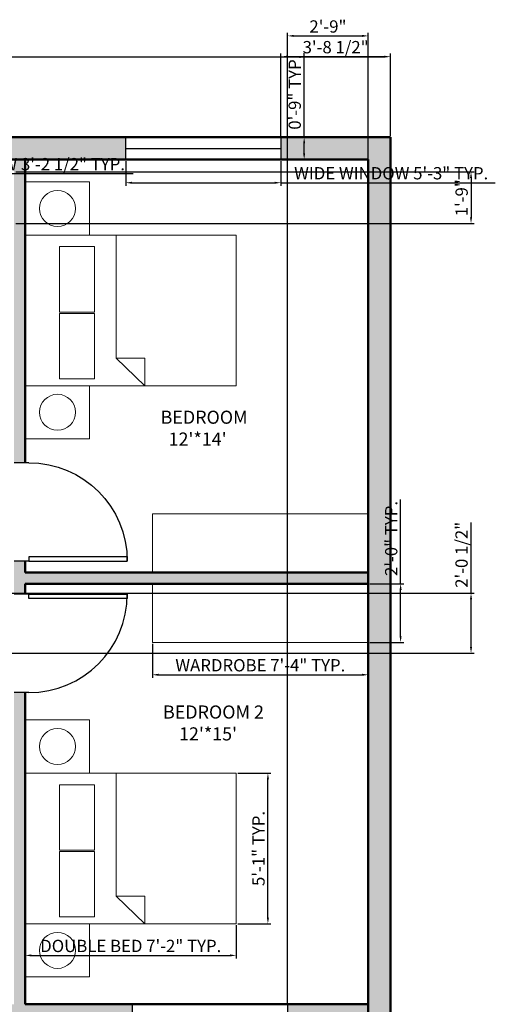
# Model space of a CAD drawing. Units: inches. Extents: x 2152 to 2718, y 1095 to 1798.
# Tile 5 of 5: x 2524 to 2718, y 1394 to 1794. Entities that reach past the tile are written whole.
import ezdxf

# ---------------------------------------------------------------- set-up
doc = ezdxf.new("R2010")
doc.units = ezdxf.units.IN
for name, color, linetype, lineweight in [('A-ANNO-DIMS', 130, 'Continuous', 18), ('A-AREA-IDEN', 130, 'Continuous', 25), ('A-FLOR-CASE', 10, 'Continuous', 20), ('A-WALL-PATT', 210, 'Continuous', 13), ('DOOR', 160, 'Continuous', 25), ('FUR', 10, 'Continuous', 18), ('WALL', 7, 'Continuous', 50), ('WIND', 140, 'Continuous', 25)]:
    doc.layers.add(name, color=color, linetype=linetype, lineweight=lineweight)
doc.styles.get("Standard").update_dxf_attribs({"font": 'arial.ttf'})
doc.dimstyles.new('ISO-25', dxfattribs={"dimtxt": 5, "dimasz": 2.5, "dimexe": 1.25, "dimexo": 0.625, "dimtad": 1, "dimdec": 0, "dimlunit": 4, "dimtxsty": 'Standard', "dimcen": 2.5, "dimadec": 0, "dimazin": 0, "dimtfac": 1, "dimtdec": 0, "dimtmove": 0, "dimatfit": 3, "dimfxl": 1, "dimarcsym": 0})

# ---------------------------------------------------------------- blocks, each defined once
blk = doc.blocks.new('*U2')
for p, q in [((0, 0), (0, -6)), ((40, 0), (40, -6))]:
    blk.add_line(p, q)
blk.add_lwpolyline([(0, 0), (0, 40), (1.75, 40), (1.75, 0)], close=True)
blk.add_arc((0, 0), 40, 0, 90)
blk = doc.blocks.new('*D13')
at = {"layer": 'A-ANNO-DIMS', "color": 0, "lineweight": -2, "transparency": 16777216}
for p, q in [((2195.06, 1746.99), (2195.06, 1780.4)), ((2197.56, 1779.15), (2672.56, 1779.15)), ((2675.06, 1746.99), (2675.06, 1780.4))]:
    blk.add_line(p, q, dxfattribs=at)
at = {"layer": 'A-ANNO-DIMS', "color": 0, "transparency": 16777216}
for points in [[(2197.56, 1779.57), (2197.56, 1778.74), (2195.06, 1779.15)], [(2672.56, 1779.57), (2672.56, 1778.74), (2675.06, 1779.15)]]:
    blk.add_solid(points, dxfattribs=at)
at = {"layer": 'Defpoints', "color": 0, "transparency": 16777216}
for p in [(2675.06, 1779.15), (2195.06, 1746.37), (2675.06, 1746.37)]:
    blk.add_point(p, dxfattribs=at)
at = {"layer": 'A-ANNO-DIMS', "color": 0, "transparency": 16777216, "insert": (2435.06, 1782.33), "char_height": 5, "attachment_point": 5}
blk.add_mtext("40'", dxfattribs=at)
blk = doc.blocks.new('WIN-WIDE')
blk.add_line((0, 4.5), (63.07, 4.5))
blk.add_lwpolyline([(0, 9), (63.07, 9), (63.07, 0), (0, 0)], close=True)
blk = doc.blocks.new('BED-DOUBLE')
for p, q in [((37.05, 61.24), (37.05, 11.23)), ((37.05, 11.23), (48.59, 11.23)), ((48.59, 0), (37.05, 11.23)), ((48.59, 11.23), (48.59, 0))]:
    blk.add_line(p, q)
for points in [[(0, 61.24), (85.82, 61.24), (85.82, 0), (0, 0)], [(13.94, 29.93), (28.11, 29.93), (28.11, 56.53), (13.94, 56.53)], [(13.94, 2.81), (28.11, 2.81), (28.11, 29.41), (13.94, 29.41)]]:
    blk.add_lwpolyline(points, close=True)
blk = doc.blocks.new('NIGHTSTAND')
blk.add_lwpolyline([(0, 21.63), (26.19, 21.63), (26.19, 0), (0, 0)], close=True)
blk.add_circle((13.1, 10.82), 7.32)
blk = doc.blocks.new('WARDROBE')
blk.add_lwpolyline([(0, 0), (87.78, 0), (87.78, 23.85), (0, 23.85)], close=True)
blk = doc.blocks.new('*D24')
at = {"layer": 'A-ANNO-DIMS', "color": 0, "lineweight": -2, "transparency": 16777216}
for p, q in [((2567.46, 1736.74), (2567.46, 1726.66)), ((2630.54, 1736.74), (2630.54, 1726.66)), ((2569.96, 1727.91), (2628.04, 1727.91)), ((2630.54, 1727.91), (2717.74, 1727.91))]:
    blk.add_line(p, q, dxfattribs=at)
at = {"layer": 'A-ANNO-DIMS', "color": 0, "transparency": 16777216}
for points in [[(2569.96, 1728.32), (2569.96, 1727.49), (2567.46, 1727.91)], [(2628.04, 1728.32), (2628.04, 1727.49), (2630.54, 1727.91)]]:
    blk.add_solid(points, dxfattribs=at)
at = {"layer": 'Defpoints', "color": 0, "transparency": 16777216}
for p in [(2567.46, 1737.37), (2630.54, 1737.37), (2630.54, 1727.91)]:
    blk.add_point(p, dxfattribs=at)
at = {"layer": 'A-ANNO-DIMS', "color": 0, "transparency": 16777216, "insert": (2675.39, 1731.12), "char_height": 5, "attachment_point": 5}
blk.add_mtext('WIDE WINDOW 5\'-3" TYP.', dxfattribs=at)
blk = doc.blocks.new('*D25')
at = {"layer": 'A-ANNO-DIMS', "color": 0, "lineweight": -2, "transparency": 16777216}
for p, q in [((2640, 1746.37), (2640, 1780.59)), ((2631.16, 1746.37), (2641.25, 1746.37)), ((2640, 1739.87), (2640, 1743.87)), ((2631.16, 1737.37), (2641.25, 1737.37))]:
    blk.add_line(p, q, dxfattribs=at)
at = {"layer": 'A-ANNO-DIMS', "color": 0, "transparency": 16777216}
for points in [[(2639.58, 1743.87), (2640.42, 1743.87), (2640, 1746.37)], [(2639.58, 1739.87), (2640.42, 1739.87), (2640, 1737.37)]]:
    blk.add_solid(points, dxfattribs=at)
at = {"layer": 'Defpoints', "color": 0, "transparency": 16777216}
for p in [(2630.54, 1746.37), (2640, 1746.37), (2630.54, 1737.37)]:
    blk.add_point(p, dxfattribs=at)
at = {"layer": 'A-ANNO-DIMS', "color": 0, "transparency": 16777216, "insert": (2636.82, 1764.73), "char_height": 5, "attachment_point": 5, "rotation": 90}
blk.add_mtext('0\'-9" TYP.', dxfattribs=at)
blk = doc.blocks.new('*D26')
at = {"layer": 'A-ANNO-DIMS', "color": 0, "lineweight": -2, "transparency": 16777216}
for p, q in [((2420.03, 1736.74), (2420.03, 1730.35)), ((2458.48, 1736.74), (2458.48, 1730.35)), ((2422.53, 1731.6), (2455.98, 1731.6)), ((2458.48, 1731.6), (2570.46, 1731.6))]:
    blk.add_line(p, q, dxfattribs=at)
at = {"layer": 'A-ANNO-DIMS', "color": 0, "transparency": 16777216}
for points in [[(2422.53, 1732.02), (2422.53, 1731.18), (2420.03, 1731.6)], [(2455.98, 1732.02), (2455.98, 1731.18), (2458.48, 1731.6)]]:
    blk.add_solid(points, dxfattribs=at)
at = {"layer": 'Defpoints', "color": 0, "transparency": 16777216}
for p in [(2420.03, 1737.37), (2458.48, 1737.37), (2458.48, 1731.6)]:
    blk.add_point(p, dxfattribs=at)
at = {"layer": 'A-ANNO-DIMS', "color": 0, "transparency": 16777216, "insert": (2515.72, 1734.81), "char_height": 5, "attachment_point": 5}
blk.add_mtext('NARROW WINDOW 3\'-2 1/2" TYP.', dxfattribs=at)
blk = doc.blocks.new('*D28')
at = {"layer": 'A-ANNO-DIMS', "color": 0, "lineweight": -2, "transparency": 16777216}
for p, q in [((2526.56, 1425.99), (2526.56, 1412.49)), ((2612.38, 1425.99), (2612.38, 1412.49)), ((2529.06, 1413.74), (2609.88, 1413.74))]:
    blk.add_line(p, q, dxfattribs=at)
at = {"layer": 'A-ANNO-DIMS', "color": 0, "transparency": 16777216}
for points in [[(2529.06, 1414.16), (2529.06, 1413.33), (2526.56, 1413.74)], [(2609.88, 1414.16), (2609.88, 1413.33), (2612.38, 1413.74)]]:
    blk.add_solid(points, dxfattribs=at)
at = {"layer": 'Defpoints', "color": 0, "transparency": 16777216}
for p in [(2526.56, 1426.61), (2612.38, 1426.61), (2612.38, 1413.74)]:
    blk.add_point(p, dxfattribs=at)
at = {"layer": 'A-ANNO-DIMS', "color": 0, "transparency": 16777216, "insert": (2569.47, 1416.95), "char_height": 5, "attachment_point": 5}
blk.add_mtext('DOUBLE BED 7\'-2" TYP.', dxfattribs=at)
blk = doc.blocks.new('*D29')
at = {"layer": 'A-ANNO-DIMS', "color": 0, "lineweight": -2, "transparency": 16777216}
for p, q in [((2613, 1487.86), (2626.5, 1487.86)), ((2625.25, 1429.11), (2625.25, 1485.36)), ((2613, 1426.61), (2626.5, 1426.61))]:
    blk.add_line(p, q, dxfattribs=at)
at = {"layer": 'A-ANNO-DIMS', "color": 0, "transparency": 16777216}
for points in [[(2624.84, 1485.36), (2625.67, 1485.36), (2625.25, 1487.86)], [(2624.84, 1429.11), (2625.67, 1429.11), (2625.25, 1426.61)]]:
    blk.add_solid(points, dxfattribs=at)
at = {"layer": 'Defpoints', "color": 0, "transparency": 16777216}
for p in [(2612.38, 1487.86), (2625.25, 1487.86), (2612.38, 1426.61)]:
    blk.add_point(p, dxfattribs=at)
at = {"layer": 'A-ANNO-DIMS', "color": 0, "transparency": 16777216, "insert": (2622.07, 1457.23), "char_height": 5, "attachment_point": 5, "rotation": 90}
blk.add_mtext('5\'-1" TYP.', dxfattribs=at)
blk = doc.blocks.new('*D34')
at = {"layer": 'A-ANNO-DIMS', "color": 0, "lineweight": -2, "transparency": 16777216}
for p, q in [((2578.28, 1540.39), (2578.28, 1526.6)), ((2666.06, 1540.39), (2666.06, 1526.6)), ((2580.78, 1527.85), (2663.56, 1527.85))]:
    blk.add_line(p, q, dxfattribs=at)
at = {"layer": 'A-ANNO-DIMS', "color": 0, "transparency": 16777216}
for points in [[(2580.78, 1528.27), (2580.78, 1527.43), (2578.28, 1527.85)], [(2663.56, 1528.27), (2663.56, 1527.43), (2666.06, 1527.85)]]:
    blk.add_solid(points, dxfattribs=at)
at = {"layer": 'Defpoints', "color": 0, "transparency": 16777216}
for p in [(2578.28, 1541.02), (2666.06, 1541.02), (2666.06, 1527.85)]:
    blk.add_point(p, dxfattribs=at)
at = {"layer": 'A-ANNO-DIMS', "color": 0, "transparency": 16777216, "insert": (2622.17, 1531.06), "char_height": 5, "attachment_point": 5}
blk.add_mtext('WARDROBE 7\'-4" TYP.', dxfattribs=at)
blk = doc.blocks.new('*D35')
at = {"layer": 'A-ANNO-DIMS', "color": 0, "lineweight": -2, "transparency": 16777216}
for p, q in [((2679.23, 1564.87), (2679.23, 1599.18)), ((2666.68, 1564.87), (2680.48, 1564.87)), ((2679.23, 1543.52), (2679.23, 1562.37)), ((2666.68, 1541.02), (2680.48, 1541.02))]:
    blk.add_line(p, q, dxfattribs=at)
at = {"layer": 'A-ANNO-DIMS', "color": 0, "transparency": 16777216}
for points in [[(2678.81, 1562.37), (2679.64, 1562.37), (2679.23, 1564.87)], [(2678.81, 1543.52), (2679.64, 1543.52), (2679.23, 1541.02)]]:
    blk.add_solid(points, dxfattribs=at)
at = {"layer": 'Defpoints', "color": 0, "transparency": 16777216}
for p in [(2666.06, 1564.87), (2679.23, 1564.87), (2666.06, 1541.02)]:
    blk.add_point(p, dxfattribs=at)
at = {"layer": 'A-ANNO-DIMS', "color": 0, "transparency": 16777216, "insert": (2676.05, 1583.27), "char_height": 5, "attachment_point": 5, "rotation": 90}
blk.add_mtext('2\'-0" TYP.', dxfattribs=at)
blk = doc.blocks.new('*D39')
at = {"layer": 'A-ANNO-DIMS', "color": 0, "lineweight": -2, "transparency": 16777216}
for p, q in [((2630.54, 1746.99), (2630.54, 1780.42)), ((2633.04, 1779.17), (2672.56, 1779.17)), ((2675.06, 1746.99), (2675.06, 1780.42))]:
    blk.add_line(p, q, dxfattribs=at)
at = {"layer": 'A-ANNO-DIMS', "color": 0, "transparency": 16777216}
for points in [[(2633.04, 1779.58), (2633.04, 1778.75), (2630.54, 1779.17)], [(2672.56, 1779.58), (2672.56, 1778.75), (2675.06, 1779.17)]]:
    blk.add_solid(points, dxfattribs=at)
at = {"layer": 'Defpoints', "color": 0, "transparency": 16777216}
for p in [(2675.06, 1779.17), (2630.54, 1746.37), (2675.06, 1746.37)]:
    blk.add_point(p, dxfattribs=at)
at = {"layer": 'A-ANNO-DIMS', "color": 0, "transparency": 16777216, "insert": (2652.8, 1782.38), "char_height": 5, "attachment_point": 5}
blk.add_mtext('3\'-8 1/2"', dxfattribs=at)
blk = doc.blocks.new('*D44')
at = {"layer": 'A-ANNO-DIMS', "color": 0, "lineweight": -2, "transparency": 16777216}
for p, q in [((2633.28, 1394.49), (2633.28, 1788.86)), ((2635.78, 1787.61), (2663.56, 1787.61)), ((2666.06, 1394.49), (2666.06, 1788.86))]:
    blk.add_line(p, q, dxfattribs=at)
at = {"layer": 'A-ANNO-DIMS', "color": 0, "transparency": 16777216}
for points in [[(2635.78, 1788.03), (2635.78, 1787.19), (2633.28, 1787.61)], [(2663.56, 1788.03), (2663.56, 1787.19), (2666.06, 1787.61)]]:
    blk.add_solid(points, dxfattribs=at)
at = {"layer": 'Defpoints', "color": 0, "transparency": 16777216}
for p in [(2666.06, 1787.61), (2633.28, 1393.87), (2666.06, 1393.87)]:
    blk.add_point(p, dxfattribs=at)
at = {"layer": 'A-ANNO-DIMS', "color": 0, "transparency": 16777216, "insert": (2649.67, 1790.79), "char_height": 5, "attachment_point": 5}
blk.add_mtext('2\'-9"', dxfattribs=at)
blk = doc.blocks.new('*D50')
at = {"layer": 'A-ANNO-DIMS', "color": 0, "lineweight": -2, "transparency": 16777216}
for p, q in [((2707.86, 1560.98), (2707.86, 1589.76)), ((2281.18, 1560.98), (2709.11, 1560.98)), ((2707.86, 1539.09), (2707.86, 1558.48)), ((2281.18, 1536.59), (2709.11, 1536.59))]:
    blk.add_line(p, q, dxfattribs=at)
at = {"layer": 'A-ANNO-DIMS', "color": 0, "transparency": 16777216}
for points in [[(2707.44, 1558.48), (2708.28, 1558.48), (2707.86, 1560.98)], [(2707.44, 1539.09), (2708.28, 1539.09), (2707.86, 1536.59)]]:
    blk.add_solid(points, dxfattribs=at)
at = {"layer": 'Defpoints', "color": 0, "transparency": 16777216}
for p in [(2280.56, 1560.98), (2707.86, 1560.98), (2280.56, 1536.59)]:
    blk.add_point(p, dxfattribs=at)
at = {"layer": 'A-ANNO-DIMS', "color": 0, "transparency": 16777216, "insert": (2704.65, 1576.62), "char_height": 5, "attachment_point": 5, "rotation": 90}
blk.add_mtext('2\'-0 1/2"', dxfattribs=at)
blk = doc.blocks.new('*D58')
at = {"layer": 'A-ANNO-DIMS', "color": 0, "lineweight": -2, "transparency": 16777216}
for p, q in [((2522.68, 1732.31), (2709.11, 1732.31)), ((2707.86, 1729.81), (2707.86, 1713.81)), ((2522.68, 1711.31), (2709.11, 1711.31))]:
    blk.add_line(p, q, dxfattribs=at)
at = {"layer": 'A-ANNO-DIMS', "color": 0, "transparency": 16777216}
for points in [[(2707.44, 1729.81), (2708.28, 1729.81), (2707.86, 1732.31)], [(2707.44, 1713.81), (2708.28, 1713.81), (2707.86, 1711.31)]]:
    blk.add_solid(points, dxfattribs=at)
at = {"layer": 'Defpoints', "color": 0, "transparency": 16777216}
for p in [(2522.06, 1732.31), (2522.06, 1711.31), (2707.86, 1711.31)]:
    blk.add_point(p, dxfattribs=at)
at = {"layer": 'A-ANNO-DIMS', "color": 0, "transparency": 16777216, "insert": (2704.68, 1721.81), "char_height": 5, "attachment_point": 5, "rotation": 90}
blk.add_mtext('1\'-9"', dxfattribs=at)

msp = doc.modelspace()

# ---------------------------------------------------------------- hatches: boundary and pattern name
at = {"layer": 'A-WALL-PATT'}
h = msp.add_hatch(color=256, dxfattribs=at)
h.dxf.hatch_style = 1
h.paths.add_polyline_path([(2204.06, 1737.37), (2275.93, 1737.37), (2275.93, 1746.37), (2195.06, 1746.37), (2195.06, 1548.16), (2204.06, 1548.16)])
h.paths.add_polyline_path([(2567.46, 1746.37), (2519.79, 1746.37), (2519.79, 1737.37), (2549.06, 1737.37), (2567.46, 1737.37)])
h.paths.add_polyline_path([(2526.56, 1706.63), (2526.56, 1737.37), (2522.06, 1737.37), (2522.06, 1614.04), (2526.56, 1614.04), (2526.56, 1660.87)])
h.paths.add_polyline_path([(2477.06, 1737.37), (2472.56, 1737.37), (2472.56, 1653.37), (2430.09, 1653.37), (2430.09, 1648.87), (2472.56, 1648.87), (2472.56, 1569.37), (2400.56, 1569.37), (2400.56, 1573.72), (2399.94, 1573.72), (2396.06, 1573.72), (2396.06, 1569.37), (2393.45, 1569.37), (2393.45, 1564.87), (2477.06, 1564.87), (2477.06, 1648.87)])
h.paths.add_polyline_path([(2400.56, 1737.37), (2396.06, 1737.37), (2396.06, 1599.61), (2400.56, 1599.61), (2400.56, 1648.87), (2402.42, 1648.87), (2402.42, 1653.37), (2400.56, 1653.37)], flags=17)
h.paths.add_polyline_path([(2353.45, 1569.37), (2204.06, 1569.37), (2204.06, 1564.87), (2353.45, 1564.87)])
h.paths.add_polyline_path([(2280.56, 1492.87), (2221.07, 1492.87), (2221.07, 1488.37), (2280.56, 1488.37)])
h.paths.add_polyline_path([(2221.07, 1492.87), (2204.06, 1492.87), (2204.06, 1488.37), (2221.07, 1488.37)])
h.paths.add_polyline_path([(2280.56, 1536.59), (2276.9, 1536.59, -0.008622), (2276.06, 1536.6), (2276.06, 1492.87), (2280.56, 1492.87)])
h.paths.add_polyline_path([(2280.56, 1564.87), (2276.06, 1564.87), (2276.06, 1560.98), (2276.9, 1560.98), (2280.56, 1560.98)])
h.paths.add_polyline_path([(2675.06, 1746.37), (2630.54, 1746.37), (2630.54, 1737.37), (2666.06, 1737.37), (2666.06, 1384.87), (2675.06, 1384.87)])
h.paths.add_polyline_path([(2666.06, 1569.37), (2578.28, 1569.37), (2526.56, 1569.37), (2526.56, 1574.04), (2522.06, 1574.04), (2522.06, 1564.87), (2522.06, 1560.6), (2526.56, 1560.6), (2526.56, 1564.87), (2666.06, 1564.87)])
h.paths.add_polyline_path([(2526.56, 1520.6), (2522.06, 1520.6), (2522.06, 1384.87), (2570.2, 1384.87), (2570.2, 1393.87), (2526.56, 1393.87)])
h.paths.add_polyline_path([(2666.06, 1393.87), (2633.28, 1393.87), (2633.28, 1384.87), (2666.06, 1384.87)], flags=17)
h.paths.add_polyline_path([(2522.06, 1393.87), (2306.06, 1393.87), (2280.56, 1393.87), (2280.56, 1384.87), (2301.56, 1384.87), (2522.06, 1384.87)])
h.paths.add_polyline_path([(2280.56, 1393.87), (2204.06, 1393.87), (2204.06, 1384.87), (2232.43, 1384.87), (2280.56, 1384.87)])
h.paths.add_polyline_path([(2204.06, 1509.71), (2195.06, 1509.71), (2195.06, 1364.72), (2204.06, 1364.72), (2204.06, 1384.87)])
h.paths.add_polyline_path([(2204.06, 1326.27), (2195.06, 1326.27), (2195.06, 1302.62), (2201.06, 1302.62), (2204.06, 1302.62), (2204.06, 1308.37)])
h.paths.add_polyline_path([(2280.56, 1384.87), (2276.06, 1384.87), (2276.06, 1312.87), (2273.63, 1312.87), (2273.63, 1312.11), (2273.63, 1308.37), (2280.56, 1308.37)])
h.paths.add_polyline_path([(2248.67, 1312.11, -0.007577), (2248.69, 1312.87), (2204.06, 1312.87), (2204.06, 1308.37), (2248.67, 1308.37)])
h.paths.add_polyline_path([(2364.43, 1297.87), (2364.43, 1300.87), (2357.06, 1300.87), (2357.06, 1291.87), (2364.43, 1291.87)])
h.paths.add_polyline_path([(2428.34, 1300.87), (2404.32, 1300.87, -0.01877), (2404.43, 1297.87), (2404.43, 1291.87), (2428.34, 1291.87)])
h.paths.add_polyline_path([(2522.06, 1384.87), (2513.06, 1384.87), (2513.06, 1300.87), (2491.42, 1300.87), (2491.42, 1291.87), (2522.06, 1291.87)])
h.paths.add_polyline_path([(2357.06, 1384.87), (2348.06, 1384.87), (2348.06, 1176.37), (2309.1, 1176.37), (2309.1, 1167.37), (2357.06, 1167.37), (2357.06, 1173.65)])
h.paths.add_polyline_path([(2475.5, 1693.24), (2504.24, 1693.24), (2504.24, 1713.14), (2475.5, 1713.14)], flags=9)

# ---------------------------------------------------------------- linework, layer by layer
at = {"layer": 'WALL'}
for p, q in [((2195.06, 1746.37), (2675.06, 1746.37)), ((2675.06, 1746.37), (2675.06, 1384.87)), ((2204.06, 1737.37), (2666.06, 1737.37)), ((2477.06, 1737.37), (2549.06, 1737.37)), ((2526.56, 1737.37), (2526.56, 1660.87)), ((2553.56, 1737.37), (2666.06, 1737.37)), ((2666.06, 1737.37), (2666.06, 1164.22)), ((2526.56, 1660.87), (2526.56, 1614.04)), ((2526.56, 1574.04), (2526.56, 1569.37)), ((2526.56, 1569.37), (2666.06, 1569.37)), ((2526.56, 1564.87), (2666.06, 1564.87)), ((2526.56, 1560.6), (2526.56, 1564.87)), ((2666.06, 1564.87), (2666.06, 1384.87)), ((2526.56, 1393.87), (2526.56, 1520.6)), ((2666.06, 1393.87), (2526.56, 1393.87))]:
    msp.add_line(p, q, dxfattribs=at)

# ---------------------------------------------------------------- block references
at = {"layer": 'A-FLOR-CASE'}
for p in [(2578.28, 1569.37), (2578.28, 1541.02)]:
    msp.add_blockref('WARDROBE', p, dxfattribs=at)
at = {"layer": 'DOOR', "xscale": -1, "rotation": 270}
msp.add_blockref('*U2', (2528.06, 1574.04), dxfattribs=at)
at = {"layer": 'DOOR', "rotation": 270}
msp.add_blockref('*U2', (2528.06, 1560.6), dxfattribs=at)
at = {"layer": 'FUR'}
for name, p in [('NIGHTSTAND', (2526.56, 1706.63)), ('BED-DOUBLE', (2526.56, 1645.39)), ('NIGHTSTAND', (2526.56, 1623.76)), ('NIGHTSTAND', (2526.56, 1487.86)), ('BED-DOUBLE', (2526.56, 1426.62)), ('NIGHTSTAND', (2526.56, 1404.98))]:
    msp.add_blockref(name, p, dxfattribs=at)
at = {"layer": 'WIND'}
for p in [(2567.46, 1737.37), (2570.2, 1384.87)]:
    msp.add_blockref('WIN-WIDE', p, dxfattribs=at)

# ---------------------------------------------------------------- texts
at = {"layer": 'A-AREA-IDEN', "attachment_point": 1}
for s, insert, char_height in [("BEDROOM\\P  12'*14'", (2581.62, 1635.23), 5.331), ("BEDROOM 2\\P    12'*15'", (2582.6, 1515.37), 5.3311)]:
    msp.add_mtext_dynamic_manual_height_columns(s, width=138.497, gutter_width=26.66, heights=[0], dxfattribs=dict(at, insert=insert, char_height=char_height))

# ---------------------------------------------------------------- dimensions: what is measured, and where the dimension line sits
at = {"layer": 'A-ANNO-DIMS'}
for base, p1, p2, override, picture, middle in [((2666.06, 1787.61), (2633.28, 1393.87), (2666.06, 1393.87), {"dimdec": 1, "dimlfac": 1, "dimrnd": 0, "dimzin": 1, "dimdsep": 46, "dimlunit": 4, "dimfrac": 2}, '*D44', (2649.67, 1790.79)), ((2675.06, 1779.15), (2195.06, 1746.37), (2675.06, 1746.37), {"dimclrd": 0, "dimclre": 0, "dimclrt": 0}, '*D13', (2435.06, 1782.33))]:
    dim = msp.add_linear_dim(base=base, p1=p1, p2=p2, dimstyle='ISO-25', override=override, dxfattribs=at)
    dim.commit()
    dim.dimension.update_dxf_attribs({"geometry": picture, "text_midpoint": middle})
for base, p1, p2, angle, picture, middle in [((2675.06, 1779.17), (2630.54, 1746.37), (2675.06, 1746.37), 0, '*D39', (2652.8, 1782.38)), ((2707.86, 1711.31), (2522.06, 1732.31), (2522.06, 1711.31), 90, '*D58', (2704.68, 1721.81)), ((2707.86, 1560.98), (2280.56, 1536.59), (2280.56, 1560.98), 90, '*D50', (2704.65, 1576.62))]:
    dim = msp.add_linear_dim(base=base, p1=p1, p2=p2, angle=angle, dimstyle='ISO-25', override={"dimdec": 1, "dimlfac": 1, "dimrnd": 0, "dimzin": 1, "dimdsep": 46, "dimlunit": 4, "dimfrac": 2}, dxfattribs=at)
    dim.commit()
    dim.dimension.update_dxf_attribs({"geometry": picture, "text_midpoint": middle})
for base, p1, p2, picture, middle in [((2640, 1746.37), (2630.54, 1737.37), (2630.54, 1746.37), '*D25', (2636.82, 1764.73)), ((2679.2259, 1564.8669), (2666.0592, 1541.0175), (2666.0592, 1564.8669), '*D35', (2676.048, 1583.2733)), ((2625.2518, 1487.8551), (2612.3788, 1426.6148), (2612.3788, 1487.8551), '*D29', (2622.0739, 1457.235))]:
    dim = msp.add_linear_dim(base=base, p1=p1, p2=p2, angle=90, text='<> TYP.', dimstyle='ISO-25', override={"dimdec": 1, "dimlfac": 1, "dimrnd": 0, "dimzin": 1, "dimdsep": 46, "dimlunit": 4, "dimfrac": 2}, dxfattribs=at)
    dim.commit()
    dim.dimension.update_dxf_attribs({"geometry": picture, "text_midpoint": middle})
for base, p1, p2, text, picture, middle in [((2458.4762, 1731.6002), (2420.0312, 1737.3669), (2458.4762, 1737.3669), 'NARROW WINDOW <> TYP.', '*D26', (2515.7178, 1734.8138)), ((2630.54, 1727.91), (2567.46, 1737.37), (2630.54, 1737.37), 'WIDE WINDOW <> TYP.', '*D24', (2675.39, 1731.12)), ((2666.06, 1527.85), (2578.28, 1541.02), (2666.06, 1541.02), 'WARDROBE <> TYP.', '*D34', (2622.17, 1531.06)), ((2612.38, 1413.74), (2526.56, 1426.61), (2612.38, 1426.61), 'DOUBLE BED <> TYP.', '*D28', (2569.47, 1416.95))]:
    dim = msp.add_linear_dim(base=base, p1=p1, p2=p2, text=text, dimstyle='ISO-25', override={"dimdec": 1, "dimlfac": 1, "dimrnd": 0, "dimzin": 1, "dimdsep": 46, "dimlunit": 4, "dimfrac": 2}, dxfattribs=at)
    dim.commit()
    dim.dimension.update_dxf_attribs({"geometry": picture, "text_midpoint": middle})

doc.saveas('drawing.dxf')
